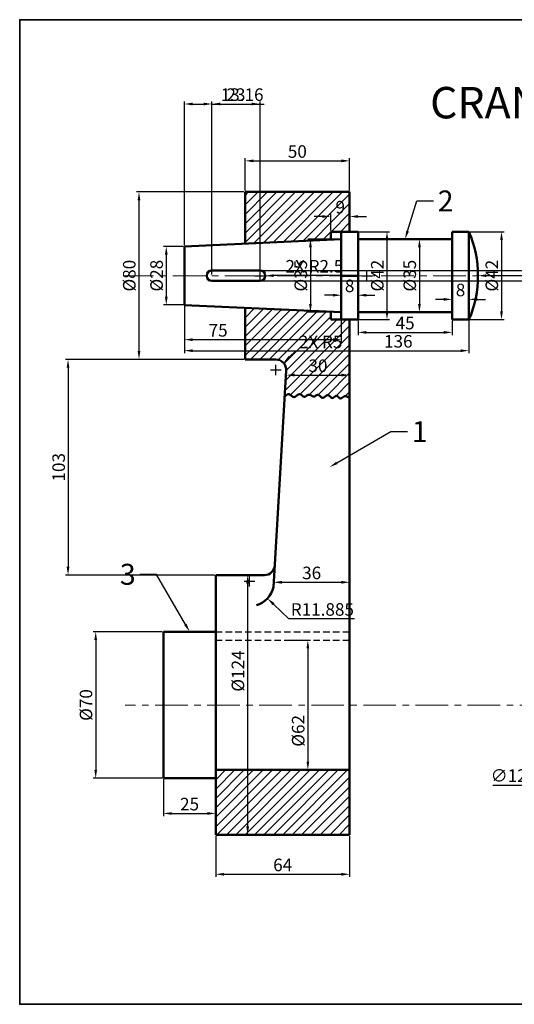
# Model space of a CAD drawing. Units: millimetres. Extents: x -165 to 405, y -25 to 445.
# Tile 1 of 2: x -165 to 72, y -25 to 445. Entities that reach past the tile are written whole.
import ezdxf
from ezdxf import colors
from ezdxf.entities.mleader import LeaderData, LeaderLine
from ezdxf.math import Vec2, Vec3

# ---------------------------------------------------------------- set-up
doc = ezdxf.new("R2010")
doc.units = ezdxf.units.MM
doc.header["$LTSCALE"] = 0.7
doc.linetypes.add('CENTER', pattern=[50.8, 31.75, -6.35, 6.35, -6.35])
doc.linetypes.add('HIDDEN', pattern=[9.525, 6.35, -3.175])
for name, color, linetype, lineweight in [('M-CNTR', 1, 'CENTER', 18), ('M-DIMS', 2, 'Continuous', 25), ('M-HATC', 8, 'Continuous', 18), ('M-HIDN', 6, 'HIDDEN', 25), ('M-OUTL', 7, 'Continuous', 50), ('M-TEXT', 3, 'Continuous', 25), ('M-TTLB', 7, 'Continuous', 35)]:
    doc.layers.add(name, color=color, linetype=linetype, lineweight=lineweight)
doc.styles.get("Standard").update_dxf_attribs({"font": 'arial.ttf'})
doc.dimstyles.new('ISO-25', dxfattribs={"dimtxt": 6, "dimasz": 4, "dimexe": 1.25, "dimexo": 0.625, "dimtad": 1, "dimtoh": 1, "dimdec": 0, "dimtxsty": 'Standard', "dimcen": 2.5, "dimadec": 0, "dimazin": 0, "dimtfac": 1, "dimtdec": 0, "dimtofl": 0, "dimtmove": 0, "dimatfit": 3, "dimfxl": 1, "dimarcsym": 0})

# ---------------------------------------------------------------- blocks, each defined once
blk = doc.blocks.new('*D10')
at = {"layer": 'Defpoints', "color": 0, "ltscale": 0.7, "transparency": 16777216}
for p in [(210.34, 146.19), (100.41, 88.8)]:
    blk.add_point(p, dxfattribs=at)
at = {"layer": 'M-DIMS', "color": 0, "lineweight": -2, "ltscale": 0.7, "transparency": 16777216}
for p, q in [((155.38, 115), (155.38, 120)), ((152.88, 117.5), (157.88, 117.5)), ((81.97, 79.17), (96.87, 86.95)), ((61.58, 79.17), (81.97, 79.17))]:
    blk.add_line(p, q, dxfattribs=at)
at = {"layer": 'M-DIMS', "color": 0, "ltscale": 0.7, "transparency": 16777216}
blk.add_solid([(96.56, 87.54), (97.18, 86.36), (100.41, 88.8)], dxfattribs=at)
at = {"layer": 'M-DIMS', "color": 0, "ltscale": 0.7, "transparency": 16777216, "insert": (71.46, 83.03), "char_height": 6, "attachment_point": 5}
blk.add_mtext('∅124', dxfattribs=at)
blk = doc.blocks.new('*D14')
at = {"layer": 'Defpoints', "color": 0, "ltscale": 0.7, "transparency": 16777216}
for p in [(-95.82, 152.5), (-128.19, 82.5), (-95.82, 82.5)]:
    blk.add_point(p, dxfattribs=at)
at = {"layer": 'M-DIMS', "color": 0, "lineweight": -2, "ltscale": 0.7, "transparency": 16777216}
for p, q in [((-96.44, 152.5), (-129.44, 152.5)), ((-128.19, 148.5), (-128.19, 86.5)), ((-96.44, 82.5), (-129.44, 82.5))]:
    blk.add_line(p, q, dxfattribs=at)
at = {"layer": 'M-DIMS', "color": 0, "ltscale": 0.7, "transparency": 16777216}
for points in [[(-128.86, 148.5), (-127.53, 148.5), (-128.19, 152.5)], [(-128.86, 86.5), (-127.53, 86.5), (-128.19, 82.5)]]:
    blk.add_solid(points, dxfattribs=at)
at = {"layer": 'M-DIMS', "color": 0, "ltscale": 0.7, "transparency": 16777216, "insert": (-132.05, 117.5), "char_height": 6, "attachment_point": 5, "rotation": 90}
blk.add_mtext('%%C70', dxfattribs=at)
blk = doc.blocks.new('*D15')
at = {"layer": 'Defpoints', "color": 0, "ltscale": 0.7, "transparency": 16777216}
for p in [(-95.82, 82.5), (-70.82, 82.5), (-70.82, 65.72)]:
    blk.add_point(p, dxfattribs=at)
at = {"layer": 'M-DIMS', "color": 0, "lineweight": -2, "ltscale": 0.7, "transparency": 16777216}
for p, q in [((-95.82, 81.87), (-95.82, 64.47)), ((-70.82, 81.87), (-70.82, 64.47)), ((-91.82, 65.72), (-74.82, 65.72))]:
    blk.add_line(p, q, dxfattribs=at)
at = {"layer": 'M-DIMS', "color": 0, "ltscale": 0.7, "transparency": 16777216}
for points in [[(-91.82, 66.38), (-91.82, 65.05), (-95.82, 65.72)], [(-74.82, 66.38), (-74.82, 65.05), (-70.82, 65.72)]]:
    blk.add_solid(points, dxfattribs=at)
at = {"layer": 'M-DIMS', "color": 0, "ltscale": 0.7, "transparency": 16777216, "insert": (-83.32, 69.4), "char_height": 6, "attachment_point": 5}
blk.add_mtext('25', dxfattribs=at)
blk = doc.blocks.new('*D16')
at = {"layer": 'Defpoints', "color": 0, "ltscale": 0.7, "transparency": 16777216}
for p in [(-70.82, 55.5), (-6.82, 55.5), (-6.82, 36.67)]:
    blk.add_point(p, dxfattribs=at)
at = {"layer": 'M-DIMS', "color": 0, "lineweight": -2, "ltscale": 0.7, "transparency": 16777216}
for p, q in [((-70.82, 54.87), (-70.82, 35.42)), ((-6.82, 54.87), (-6.82, 35.42)), ((-66.82, 36.67), (-10.82, 36.67))]:
    blk.add_line(p, q, dxfattribs=at)
at = {"layer": 'M-DIMS', "color": 0, "ltscale": 0.7, "transparency": 16777216}
for points in [[(-66.82, 37.34), (-66.82, 36.01), (-70.82, 36.67)], [(-10.82, 37.34), (-10.82, 36.01), (-6.82, 36.67)]]:
    blk.add_solid(points, dxfattribs=at)
at = {"layer": 'M-DIMS', "color": 0, "ltscale": 0.7, "transparency": 16777216, "insert": (-38.82, 40.36), "char_height": 6, "attachment_point": 5}
blk.add_mtext('64', dxfattribs=at)
blk = doc.blocks.new('*D17')
at = {"layer": 'Defpoints', "color": 0, "ltscale": 0.7, "transparency": 16777216}
for p in [(-59.17, 179.5), (-59.17, 55.5), (-55.59, 55.5)]:
    blk.add_point(p, dxfattribs=at)
at = {"layer": 'M-DIMS', "color": 0, "lineweight": -2, "ltscale": 0.7, "transparency": 16777216}
for p, q in [((-58.55, 179.5), (-54.34, 179.5)), ((-55.59, 175.5), (-55.59, 59.5)), ((-58.55, 55.5), (-54.34, 55.5))]:
    blk.add_line(p, q, dxfattribs=at)
at = {"layer": 'M-DIMS', "color": 0, "ltscale": 0.7, "transparency": 16777216}
for points in [[(-56.25, 175.5), (-54.92, 175.5), (-55.59, 179.5)], [(-56.25, 59.5), (-54.92, 59.5), (-55.59, 55.5)]]:
    blk.add_solid(points, dxfattribs=at)
at = {"layer": 'M-DIMS', "color": 0, "ltscale": 0.7, "transparency": 16777216, "insert": (-59.44, 133.73), "char_height": 6, "attachment_point": 5, "rotation": 90}
blk.add_mtext('%%C124', dxfattribs=at)
blk = doc.blocks.new('*D18')
at = {"layer": 'Defpoints', "color": 0, "ltscale": 0.7, "transparency": 16777216}
for p in [(-38.82, 148.5), (-38.82, 86.5), (-26.79, 86.5)]:
    blk.add_point(p, dxfattribs=at)
at = {"layer": 'M-DIMS', "color": 0, "lineweight": -2, "ltscale": 0.7, "transparency": 16777216}
for p, q in [((-38.19, 148.5), (-25.54, 148.5)), ((-26.79, 144.5), (-26.79, 90.5)), ((-38.19, 86.5), (-25.54, 86.5))]:
    blk.add_line(p, q, dxfattribs=at)
at = {"layer": 'M-DIMS', "color": 0, "ltscale": 0.7, "transparency": 16777216}
for points in [[(-27.45, 144.5), (-26.12, 144.5), (-26.79, 148.5)], [(-27.45, 90.5), (-26.12, 90.5), (-26.79, 86.5)]]:
    blk.add_solid(points, dxfattribs=at)
at = {"layer": 'M-DIMS', "color": 0, "ltscale": 0.7, "transparency": 16777216, "insert": (-30.64, 105.17), "char_height": 6, "attachment_point": 5, "rotation": 90}
blk.add_mtext('%%C62', dxfattribs=at)
blk = doc.blocks.new('*D19')
at = {"layer": 'Defpoints', "color": 0, "ltscale": 0.7, "transparency": 16777216}
for p in [(-6.82, 176.09), (-43.15, 173.79), (-6.82, 173.79)]:
    blk.add_point(p, dxfattribs=at)
at = {"layer": 'M-DIMS', "color": 0, "lineweight": -2, "ltscale": 0.7, "transparency": 16777216}
for p, q in [((-43.15, 174.41), (-43.15, 177.34)), ((-39.15, 176.09), (-10.82, 176.09)), ((-6.82, 174.41), (-6.82, 177.34))]:
    blk.add_line(p, q, dxfattribs=at)
at = {"layer": 'M-DIMS', "color": 0, "ltscale": 0.7, "transparency": 16777216}
for points in [[(-39.15, 176.76), (-39.15, 175.42), (-43.15, 176.09)], [(-10.82, 176.76), (-10.82, 175.42), (-6.82, 176.09)]]:
    blk.add_solid(points, dxfattribs=at)
at = {"layer": 'M-DIMS', "color": 0, "ltscale": 0.7, "transparency": 16777216, "insert": (-24.98, 179.78), "char_height": 6, "attachment_point": 5}
blk.add_mtext('36', dxfattribs=at)
blk = doc.blocks.new('*D20')
at = {"layer": 'Defpoints', "color": 0, "ltscale": 0.7, "transparency": 16777216}
for p in [(-37.12, 277.21), (-6.82, 277.21), (-6.82, 275.03)]:
    blk.add_point(p, dxfattribs=at)
at = {"layer": 'M-DIMS', "color": 0, "lineweight": -2, "ltscale": 0.7, "transparency": 16777216}
for p, q in [((-37.12, 276.58), (-37.12, 273.78)), ((-33.12, 275.03), (-10.82, 275.03)), ((-6.82, 276.58), (-6.82, 273.78))]:
    blk.add_line(p, q, dxfattribs=at)
at = {"layer": 'M-DIMS', "color": 0, "ltscale": 0.7, "transparency": 16777216}
for points in [[(-33.12, 275.7), (-33.12, 274.36), (-37.12, 275.03)], [(-10.82, 275.7), (-10.82, 274.36), (-6.82, 275.03)]]:
    blk.add_solid(points, dxfattribs=at)
at = {"layer": 'M-DIMS', "color": 0, "ltscale": 0.7, "transparency": 16777216, "insert": (-21.97, 278.72), "char_height": 6, "attachment_point": 5}
blk.add_mtext('30', dxfattribs=at)
blk = doc.blocks.new('*D21')
at = {"layer": 'Defpoints', "color": 0, "ltscale": 0.7, "transparency": 16777216}
for p in [(-85.82, 336.5), (-94.46, 308.5), (-85.82, 308.5)]:
    blk.add_point(p, dxfattribs=at)
at = {"layer": 'M-DIMS', "color": 0, "lineweight": -2, "ltscale": 0.7, "transparency": 16777216}
for p, q in [((-86.44, 336.5), (-95.71, 336.5)), ((-94.46, 332.5), (-94.46, 312.5)), ((-86.44, 308.5), (-95.71, 308.5))]:
    blk.add_line(p, q, dxfattribs=at)
at = {"layer": 'M-DIMS', "color": 0, "ltscale": 0.7, "transparency": 16777216}
for points in [[(-95.13, 332.5), (-93.79, 332.5), (-94.46, 336.5)], [(-95.13, 312.5), (-93.79, 312.5), (-94.46, 308.5)]]:
    blk.add_solid(points, dxfattribs=at)
at = {"layer": 'M-DIMS', "color": 0, "ltscale": 0.7, "transparency": 16777216, "insert": (-98.32, 322.5), "char_height": 6, "attachment_point": 5, "rotation": 90}
blk.add_mtext('%%C28', dxfattribs=at)
blk = doc.blocks.new('*D22')
at = {"layer": 'Defpoints', "color": 0, "ltscale": 0.7, "transparency": 16777216}
for p in [(-56.82, 362.5), (-107.5, 282.5), (-56.82, 282.5)]:
    blk.add_point(p, dxfattribs=at)
at = {"layer": 'M-DIMS', "color": 0, "lineweight": -2, "ltscale": 0.7, "transparency": 16777216}
for p, q in [((-57.44, 362.5), (-108.75, 362.5)), ((-107.5, 358.5), (-107.5, 286.5)), ((-57.44, 282.5), (-108.75, 282.5))]:
    blk.add_line(p, q, dxfattribs=at)
at = {"layer": 'M-DIMS', "color": 0, "ltscale": 0.7, "transparency": 16777216}
for points in [[(-108.17, 358.5), (-106.83, 358.5), (-107.5, 362.5)], [(-108.17, 286.5), (-106.83, 286.5), (-107.5, 282.5)]]:
    blk.add_solid(points, dxfattribs=at)
at = {"layer": 'M-DIMS', "color": 0, "ltscale": 0.7, "transparency": 16777216, "insert": (-111.36, 322.5), "char_height": 6, "attachment_point": 5, "rotation": 90}
blk.add_mtext('%%C80', dxfattribs=at)
blk = doc.blocks.new('*D23')
at = {"layer": 'Defpoints', "color": 0, "ltscale": 0.7, "transparency": 16777216}
for p in [(-6.82, 377.32), (-56.82, 362.5), (-6.82, 362.5)]:
    blk.add_point(p, dxfattribs=at)
at = {"layer": 'M-DIMS', "color": 0, "lineweight": -2, "ltscale": 0.7, "transparency": 16777216}
for p, q in [((-56.82, 363.12), (-56.82, 378.57)), ((-52.82, 377.32), (-10.82, 377.32)), ((-6.82, 363.12), (-6.82, 378.57))]:
    blk.add_line(p, q, dxfattribs=at)
at = {"layer": 'M-DIMS', "color": 0, "ltscale": 0.7, "transparency": 16777216}
for points in [[(-52.82, 377.99), (-52.82, 376.65), (-56.82, 377.32)], [(-10.82, 377.99), (-10.82, 376.65), (-6.82, 377.32)]]:
    blk.add_solid(points, dxfattribs=at)
at = {"layer": 'M-DIMS', "color": 0, "ltscale": 0.7, "transparency": 16777216, "insert": (-31.82, 381.01), "char_height": 6, "attachment_point": 5}
blk.add_mtext('50', dxfattribs=at)
blk = doc.blocks.new('*D24')
at = {"layer": 'Defpoints', "color": 0, "ltscale": 0.7, "transparency": 16777216}
for p in [(-6.82, 350.75), (-15.82, 343.5), (-6.82, 343.5)]:
    blk.add_point(p, dxfattribs=at)
at = {"layer": 'M-DIMS', "color": 0, "lineweight": -2, "ltscale": 0.7, "transparency": 16777216}
for p, q in [((-19.82, 350.75), (-23.82, 350.75)), ((-15.82, 344.12), (-15.82, 352)), ((-6.82, 344.12), (-6.82, 352)), ((-2.82, 350.75), (1.18, 350.75))]:
    blk.add_line(p, q, dxfattribs=at)
at = {"layer": 'M-DIMS', "color": 0, "ltscale": 0.7, "transparency": 16777216}
for points in [[(-19.82, 351.42), (-19.82, 350.09), (-15.82, 350.75)], [(-2.82, 351.42), (-2.82, 350.09), (-6.82, 350.75)]]:
    blk.add_solid(points, dxfattribs=at)
at = {"layer": 'M-DIMS', "color": 0, "ltscale": 0.7, "transparency": 16777216, "insert": (-11.32, 354.44), "char_height": 6, "attachment_point": 5}
blk.add_mtext('9', dxfattribs=at)
blk = doc.blocks.new('*D25')
at = {"layer": 'Defpoints', "color": 0, "ltscale": 0.7, "transparency": 16777216}
for p in [(-85.82, 308.5), (-10.82, 301.5), (-10.82, 291.95)]:
    blk.add_point(p, dxfattribs=at)
at = {"layer": 'M-DIMS', "color": 0, "lineweight": -2, "ltscale": 0.7, "transparency": 16777216}
for p, q in [((-85.82, 307.87), (-85.82, 290.7)), ((-10.82, 300.87), (-10.82, 290.7)), ((-81.82, 291.95), (-14.82, 291.95))]:
    blk.add_line(p, q, dxfattribs=at)
at = {"layer": 'M-DIMS', "color": 0, "ltscale": 0.7, "transparency": 16777216}
for points in [[(-81.82, 292.61), (-81.82, 291.28), (-85.82, 291.95)], [(-14.82, 292.61), (-14.82, 291.28), (-10.82, 291.95)]]:
    blk.add_solid(points, dxfattribs=at)
at = {"layer": 'M-DIMS', "color": 0, "ltscale": 0.7, "transparency": 16777216, "insert": (-69.68, 295.62), "char_height": 6, "attachment_point": 5}
blk.add_mtext('75', dxfattribs=at)
blk = doc.blocks.new('*D26')
at = {"layer": 'Defpoints', "color": 0, "ltscale": 0.7, "transparency": 16777216}
for p in [(-85.82, 322.5), (50.18, 322.5), (50.18, 286.68)]:
    blk.add_point(p, dxfattribs=at)
at = {"layer": 'M-DIMS', "color": 0, "lineweight": -2, "ltscale": 0.7, "transparency": 16777216}
for p, q in [((-85.82, 321.87), (-85.82, 285.43)), ((50.18, 321.87), (50.18, 285.43)), ((-81.82, 286.68), (46.18, 286.68))]:
    blk.add_line(p, q, dxfattribs=at)
at = {"layer": 'M-DIMS', "color": 0, "ltscale": 0.7, "transparency": 16777216}
for points in [[(-81.82, 287.35), (-81.82, 286.01), (-85.82, 286.68)], [(46.18, 287.35), (46.18, 286.01), (50.18, 286.68)]]:
    blk.add_solid(points, dxfattribs=at)
at = {"layer": 'M-DIMS', "color": 0, "ltscale": 0.7, "transparency": 16777216, "insert": (16.44, 290.37), "char_height": 6, "attachment_point": 5}
blk.add_mtext('136', dxfattribs=at)
blk = doc.blocks.new('*D27')
at = {"layer": 'Defpoints', "color": 0, "ltscale": 0.7, "transparency": 16777216}
for p in [(-10.82, 343.5), (-6.82, 301.5), (11.03, 301.5)]:
    blk.add_point(p, dxfattribs=at)
at = {"layer": 'M-DIMS', "color": 0, "lineweight": -2, "ltscale": 0.7, "transparency": 16777216}
for p, q in [((-10.19, 343.5), (12.28, 343.5)), ((11.03, 339.5), (11.03, 305.5)), ((-6.19, 301.5), (12.28, 301.5))]:
    blk.add_line(p, q, dxfattribs=at)
at = {"layer": 'M-DIMS', "color": 0, "ltscale": 0.7, "transparency": 16777216}
for points in [[(10.36, 339.5), (11.69, 339.5), (11.03, 343.5)], [(10.36, 305.5), (11.69, 305.5), (11.03, 301.5)]]:
    blk.add_solid(points, dxfattribs=at)
at = {"layer": 'M-DIMS', "color": 0, "ltscale": 0.7, "transparency": 16777216, "insert": (7.17, 322.5), "char_height": 6, "attachment_point": 5, "rotation": 90}
blk.add_mtext('%%C42', dxfattribs=at)
blk = doc.blocks.new('*D28')
at = {"layer": 'Defpoints', "color": 0, "ltscale": 0.7, "transparency": 16777216}
for p in [(-10.82, 313.17), (-2.82, 313.17), (-2.82, 313.17)]:
    blk.add_point(p, dxfattribs=at)
at = {"layer": 'M-DIMS', "color": 0, "lineweight": -2, "ltscale": 0.7, "transparency": 16777216}
for p, q in [((-14.82, 313.17), (-18.82, 313.17)), ((-10.82, 313.8), (-10.82, 314.42)), ((-2.82, 313.8), (-2.82, 314.42)), ((1.18, 313.17), (5.18, 313.17))]:
    blk.add_line(p, q, dxfattribs=at)
at = {"layer": 'M-DIMS', "color": 0, "ltscale": 0.7, "transparency": 16777216}
for points in [[(-14.82, 313.84), (-14.82, 312.51), (-10.82, 313.17)], [(1.18, 313.84), (1.18, 312.51), (-2.82, 313.17)]]:
    blk.add_solid(points, dxfattribs=at)
at = {"layer": 'M-DIMS', "color": 0, "ltscale": 0.7, "transparency": 16777216, "insert": (-6.82, 316.86), "char_height": 6, "attachment_point": 5}
blk.add_mtext('8', dxfattribs=at)
blk = doc.blocks.new('*D29')
at = {"layer": 'Defpoints', "color": 0, "ltscale": 0.7, "transparency": 16777216}
for p in [(-10.82, 340), (-25.55, 305), (-10.82, 305)]:
    blk.add_point(p, dxfattribs=at)
at = {"layer": 'M-DIMS', "color": 0, "lineweight": -2, "ltscale": 0.7, "transparency": 16777216}
for p, q in [((-11.44, 340), (-26.8, 340)), ((-25.55, 336), (-25.55, 309)), ((-11.44, 305), (-26.8, 305))]:
    blk.add_line(p, q, dxfattribs=at)
at = {"layer": 'M-DIMS', "color": 0, "ltscale": 0.7, "transparency": 16777216}
for points in [[(-26.22, 336), (-24.89, 336), (-25.55, 340)], [(-26.22, 309), (-24.89, 309), (-25.55, 305)]]:
    blk.add_solid(points, dxfattribs=at)
at = {"layer": 'M-DIMS', "color": 0, "ltscale": 0.7, "transparency": 16777216, "insert": (-29.41, 322.5), "char_height": 6, "attachment_point": 5, "rotation": 90}
blk.add_mtext('%%C35', dxfattribs=at)
blk = doc.blocks.new('*D30')
at = {"layer": 'Defpoints', "color": 0, "ltscale": 0.7, "transparency": 16777216}
for p in [(28.45, 340), (26.53, 305), (28.45, 305)]:
    blk.add_point(p, dxfattribs=at)
at = {"layer": 'M-DIMS', "color": 0, "lineweight": -2, "ltscale": 0.7, "transparency": 16777216}
for p, q in [((27.83, 340), (25.28, 340)), ((26.53, 336), (26.53, 309)), ((27.83, 305), (25.28, 305))]:
    blk.add_line(p, q, dxfattribs=at)
at = {"layer": 'M-DIMS', "color": 0, "ltscale": 0.7, "transparency": 16777216}
for points in [[(25.87, 336), (27.2, 336), (26.53, 340)], [(25.87, 309), (27.2, 309), (26.53, 305)]]:
    blk.add_solid(points, dxfattribs=at)
at = {"layer": 'M-DIMS', "color": 0, "ltscale": 0.7, "transparency": 16777216, "insert": (22.68, 322.5), "char_height": 6, "attachment_point": 5, "rotation": 90}
blk.add_mtext('%%C35', dxfattribs=at)
blk = doc.blocks.new('*D31')
at = {"layer": 'Defpoints', "color": 0, "ltscale": 0.7, "transparency": 16777216}
for p in [(46.18, 343.5), (46.18, 301.5), (65.76, 301.5)]:
    blk.add_point(p, dxfattribs=at)
at = {"layer": 'M-DIMS', "color": 0, "lineweight": -2, "ltscale": 0.7, "transparency": 16777216}
for p, q in [((46.81, 343.5), (67.01, 343.5)), ((65.76, 339.5), (65.76, 305.5)), ((46.81, 301.5), (67.01, 301.5))]:
    blk.add_line(p, q, dxfattribs=at)
at = {"layer": 'M-DIMS', "color": 0, "ltscale": 0.7, "transparency": 16777216}
for points in [[(65.1, 339.5), (66.43, 339.5), (65.76, 343.5)], [(65.1, 305.5), (66.43, 305.5), (65.76, 301.5)]]:
    blk.add_solid(points, dxfattribs=at)
at = {"layer": 'M-DIMS', "color": 0, "ltscale": 0.7, "transparency": 16777216, "insert": (61.91, 322.5), "char_height": 6, "attachment_point": 5, "rotation": 90}
blk.add_mtext('%%C42', dxfattribs=at)
blk = doc.blocks.new('*D32')
at = {"layer": 'Defpoints', "color": 0, "ltscale": 0.7, "transparency": 16777216}
for p in [(-2.82, 301.5), (42.18, 301.5), (42.18, 295.42)]:
    blk.add_point(p, dxfattribs=at)
at = {"layer": 'M-DIMS', "color": 0, "lineweight": -2, "ltscale": 0.7, "transparency": 16777216}
for p, q in [((-2.82, 300.87), (-2.82, 294.17)), ((42.18, 300.87), (42.18, 294.17)), ((1.18, 295.42), (38.18, 295.42))]:
    blk.add_line(p, q, dxfattribs=at)
at = {"layer": 'M-DIMS', "color": 0, "ltscale": 0.7, "transparency": 16777216}
for points in [[(1.18, 296.09), (1.18, 294.75), (-2.82, 295.42)], [(38.18, 296.09), (38.18, 294.75), (42.18, 295.42)]]:
    blk.add_solid(points, dxfattribs=at)
at = {"layer": 'M-DIMS', "color": 0, "ltscale": 0.7, "transparency": 16777216, "insert": (19.68, 299.09), "char_height": 6, "attachment_point": 5}
blk.add_mtext('45', dxfattribs=at)
blk = doc.blocks.new('*D33')
at = {"layer": 'Defpoints', "color": 0, "ltscale": 0.7, "transparency": 16777216}
for p in [(50.18, 311.19), (42.18, 301.5), (50.18, 301.5)]:
    blk.add_point(p, dxfattribs=at)
at = {"layer": 'M-DIMS', "color": 0, "lineweight": -2, "ltscale": 0.7, "transparency": 16777216}
for p, q in [((38.18, 311.19), (34.18, 311.19)), ((42.18, 302.12), (42.18, 312.44)), ((50.18, 302.12), (50.18, 312.44)), ((54.18, 311.19), (58.18, 311.19))]:
    blk.add_line(p, q, dxfattribs=at)
at = {"layer": 'M-DIMS', "color": 0, "ltscale": 0.7, "transparency": 16777216}
for points in [[(38.18, 311.86), (38.18, 310.52), (42.18, 311.19)], [(54.18, 311.86), (54.18, 310.52), (50.18, 311.19)]]:
    blk.add_solid(points, dxfattribs=at)
at = {"layer": 'M-DIMS', "color": 0, "ltscale": 0.7, "transparency": 16777216, "insert": (46.18, 314.88), "char_height": 6, "attachment_point": 5}
blk.add_mtext('8', dxfattribs=at)
blk = doc.blocks.new('*D39')
at = {"layer": 'Defpoints', "color": 0, "ltscale": 0.7, "transparency": 16777216}
for p in [(1.44, 322.5), (54.52, 322.5)]:
    blk.add_point(p, dxfattribs=at)
at = {"layer": 'M-DIMS', "color": 0, "lineweight": -2, "ltscale": 0.7, "transparency": 16777216}
for p, q in [((1.44, 320), (1.44, 325)), ((-1.06, 322.5), (3.94, 322.5)), ((86.36, 322.5), (58.52, 322.5)), ((112.99, 322.5), (86.36, 322.5))]:
    blk.add_line(p, q, dxfattribs=at)
at = {"layer": 'M-DIMS', "color": 0, "ltscale": 0.7, "transparency": 16777216}
blk.add_solid([(58.52, 323.16), (58.52, 321.83), (54.52, 322.5)], dxfattribs=at)
at = {"layer": 'M-DIMS', "color": 0, "ltscale": 0.7, "transparency": 16777216, "insert": (99.99, 326.19), "char_height": 6, "attachment_point": 5}
blk.add_mtext('R53.08', dxfattribs=at)
blk = doc.blocks.new('*D40')
at = {"layer": 'Defpoints', "color": 0, "ltscale": 0.7, "transparency": 16777216}
for p in [(-54.7, 176.56), (-46.08, 168.38)]:
    blk.add_point(p, dxfattribs=at)
at = {"layer": 'M-DIMS', "color": 0, "lineweight": -2, "ltscale": 0.7, "transparency": 16777216}
for p, q in [((-54.7, 174.06), (-54.7, 179.06)), ((-57.2, 176.56), (-52.2, 176.56)), ((-35.84, 158.66), (-43.18, 165.63)), ((-4.52, 158.66), (-35.84, 158.66))]:
    blk.add_line(p, q, dxfattribs=at)
at = {"layer": 'M-DIMS', "color": 0, "ltscale": 0.7, "transparency": 16777216}
blk.add_solid([(-42.72, 166.11), (-43.64, 165.14), (-46.08, 168.38)], dxfattribs=at)
at = {"layer": 'M-DIMS', "color": 0, "ltscale": 0.7, "transparency": 16777216, "insert": (-19.86, 162.34), "char_height": 6, "attachment_point": 5}
blk.add_mtext('R11.885', dxfattribs=at)
blk = doc.blocks.new('*D41')
at = {"layer": 'Defpoints', "color": 0, "ltscale": 0.7, "transparency": 16777216}
for p in [(-42.12, 277.5), (-38.48, 280.93)]:
    blk.add_point(p, dxfattribs=at)
at = {"layer": 'M-DIMS', "color": 0, "lineweight": -2, "ltscale": 0.7, "transparency": 16777216}
for p, q in [((-32.66, 286.42), (-35.57, 283.67)), ((-9.32, 286.42), (-32.66, 286.42)), ((-44.62, 277.5), (-39.62, 277.5)), ((-42.12, 275), (-42.12, 280))]:
    blk.add_line(p, q, dxfattribs=at)
at = {"layer": 'M-DIMS', "color": 0, "ltscale": 0.7, "transparency": 16777216}
blk.add_solid([(-36.03, 284.16), (-35.11, 283.19), (-38.48, 280.93)], dxfattribs=at)
at = {"layer": 'M-DIMS', "color": 0, "ltscale": 0.7, "transparency": 16777216, "insert": (-20.68, 290.1), "char_height": 6, "attachment_point": 5}
blk.add_mtext('2X R5', dxfattribs=at)
blk = doc.blocks.new('*D42')
at = {"layer": 'Defpoints', "color": 0, "ltscale": 0.7, "transparency": 16777216}
for p in [(-56.82, 282.5), (-141.41, 179.5), (-70.82, 179.5)]:
    blk.add_point(p, dxfattribs=at)
at = {"layer": 'M-DIMS', "color": 0, "lineweight": -2, "ltscale": 0.7, "transparency": 16777216}
for p, q in [((-57.44, 282.5), (-142.66, 282.5)), ((-141.41, 278.5), (-141.41, 183.5)), ((-71.44, 179.5), (-142.66, 179.5))]:
    blk.add_line(p, q, dxfattribs=at)
at = {"layer": 'M-DIMS', "color": 0, "ltscale": 0.7, "transparency": 16777216}
for points in [[(-142.08, 278.5), (-140.75, 278.5), (-141.41, 282.5)], [(-142.08, 183.5), (-140.75, 183.5), (-141.41, 179.5)]]:
    blk.add_solid(points, dxfattribs=at)
at = {"layer": 'M-DIMS', "color": 0, "ltscale": 0.7, "transparency": 16777216, "insert": (-145.11, 231), "char_height": 6, "attachment_point": 5, "rotation": 90}
blk.add_mtext('103', dxfattribs=at)
blk = doc.blocks.new('*D43')
at = {"layer": 'Defpoints', "color": 0, "ltscale": 0.7, "transparency": 16777216}
for p in [(-49.66, 404.47), (-72.66, 322.5), (-49.66, 322.5)]:
    blk.add_point(p, dxfattribs=at)
at = {"layer": 'M-DIMS', "color": 0, "lineweight": -2, "ltscale": 0.7, "transparency": 16777216}
for p, q in [((-72.66, 323.12), (-72.66, 405.72)), ((-68.66, 404.47), (-53.66, 404.47)), ((-49.66, 323.12), (-49.66, 405.72))]:
    blk.add_line(p, q, dxfattribs=at)
at = {"layer": 'M-DIMS', "color": 0, "ltscale": 0.7, "transparency": 16777216}
for points in [[(-68.66, 405.13), (-68.66, 403.8), (-72.66, 404.47)], [(-53.66, 405.13), (-53.66, 403.8), (-49.66, 404.47)]]:
    blk.add_solid(points, dxfattribs=at)
at = {"layer": 'M-DIMS', "color": 0, "ltscale": 0.7, "transparency": 16777216, "insert": (-61.16, 408.16), "char_height": 6, "attachment_point": 5}
blk.add_mtext('23', dxfattribs=at)
blk = doc.blocks.new('*D44')
at = {"layer": 'Defpoints', "color": 0, "ltscale": 0.7, "transparency": 16777216}
for p in [(-72.66, 404.47), (-85.82, 336.5), (-72.66, 322.5)]:
    blk.add_point(p, dxfattribs=at)
at = {"layer": 'M-DIMS', "color": 0, "lineweight": -2, "ltscale": 0.7, "transparency": 16777216}
for p, q in [((-85.82, 337.12), (-85.82, 405.72)), ((-81.82, 404.47), (-76.66, 404.47)), ((-72.66, 323.12), (-72.66, 405.72)), ((-72.66, 404.47), (-47.73, 404.47))]:
    blk.add_line(p, q, dxfattribs=at)
at = {"layer": 'M-DIMS', "color": 0, "ltscale": 0.7, "transparency": 16777216}
for points in [[(-81.82, 405.13), (-81.82, 403.8), (-85.82, 404.47)], [(-76.66, 405.13), (-76.66, 403.8), (-72.66, 404.47)]]:
    blk.add_solid(points, dxfattribs=at)
at = {"layer": 'M-DIMS', "color": 0, "ltscale": 0.7, "transparency": 16777216, "insert": (-58.19, 408.16), "char_height": 6, "attachment_point": 5}
blk.add_mtext('13.16', dxfattribs=at)
blk = doc.blocks.new('*D45')
at = {"layer": 'Defpoints', "color": 0, "ltscale": 0.7, "transparency": 16777216}
for p in [(-49.66, 325), (-49.66, 320), (403.9, 320)]:
    blk.add_point(p, dxfattribs=at)
at = {"layer": 'M-DIMS', "color": 0, "lineweight": -2, "ltscale": 0.7, "transparency": 16777216}
for p, q in [((403.9, 329), (403.9, 333)), ((-49.03, 325), (405.15, 325)), ((-49.03, 320), (405.15, 320)), ((403.9, 316), (403.9, 312)), ((403.9, 312), (399.29, 312))]:
    blk.add_line(p, q, dxfattribs=at)
at = {"layer": 'M-DIMS', "color": 0, "ltscale": 0.7, "transparency": 16777216}
for points in [[(403.23, 329), (404.56, 329), (403.9, 325)], [(403.23, 316), (404.56, 316), (403.9, 320)]]:
    blk.add_solid(points, dxfattribs=at)
at = {"layer": 'M-DIMS', "color": 0, "ltscale": 0.7, "transparency": 16777216, "insert": (401.28, 315.67), "char_height": 6, "attachment_point": 5}
blk.add_mtext('5', dxfattribs=at)
blk = doc.blocks.new('*D46')
at = {"layer": 'Defpoints', "color": 0, "ltscale": 0.7, "transparency": 16777216}
for p in [(-49.66, 322.5), (-47.16, 322.5)]:
    blk.add_point(p, dxfattribs=at)
at = {"layer": 'M-DIMS', "color": 0, "lineweight": -2, "ltscale": 0.7, "transparency": 16777216}
for p, q in [((-49.66, 320), (-49.66, 325)), ((-52.16, 322.5), (-47.16, 322.5)), ((-39.16, 322.51), (-43.16, 322.51)), ((-8.82, 322.51), (-39.16, 322.51))]:
    blk.add_line(p, q, dxfattribs=at)
at = {"layer": 'M-DIMS', "color": 0, "ltscale": 0.7, "transparency": 16777216}
blk.add_solid([(-43.16, 323.17), (-43.15, 321.84), (-47.16, 322.5)], dxfattribs=at)
at = {"layer": 'M-DIMS', "color": 0, "ltscale": 0.7, "transparency": 16777216, "insert": (-23.68, 326.2), "char_height": 6, "attachment_point": 5}
blk.add_mtext('2X R2.5', dxfattribs=at)

msp = doc.modelspace()

# ---------------------------------------------------------------- hatches: boundary and pattern name
at = {"layer": 'M-HATC', "ltscale": 0.7}
h = msp.add_hatch(dxfattribs=at)
h.set_pattern_fill('ANSI31', color=256)
h.paths.add_polyline_path([(-6.8156, 86.4959), (-70.8156, 86.4959), (-70.8156, 82.4959), (-70.8156, 55.4959), (-6.8156, 55.4959)])
h.paths.add_polyline_path([(-6.8156, 362.4959), (-56.8156, 362.4959), (-56.8156, 337.8492), (-15.8156, 339.7625), (-15.8156, 343.4959), (-10.8156, 343.4959), (-6.8156, 343.4959)])
edge = h.paths.add_edge_path()
edge.add_line((-15.8156, 305.2292), (-56.8156, 307.1425))
edge.add_line((-56.8156, 307.1425), (-56.8156, 282.4959))
edge.add_line((-56.8156, 282.4959), (-42.1153, 282.4959))
edge.add_arc((-42.1153, 277.4959), 5, -3.333851, 90, ccw=False)
edge.add_line((-37.1238, 277.2051), (-37.8464, 264.7996))
edge.add_spline(control_points=[(-37.8464, 264.7996), (-37.167, 265.4518), (-35.6482, 266.9098), (-33.2846, 263.1213), (-30.8198, 267.4001), (-28.5561, 263.5168), (-26.3917, 266.7417), (-24.0231, 263.8639), (-21.8949, 266.6713), (-19.7633, 262.6734), (-17.3242, 266.9021), (-15.1634, 262.8974), (-13.0907, 266.0872), (-11.2117, 262.8862), (-9.2278, 265.6704), (-7.6802, 264.7023), (-6.8156, 264.1614)], knot_values=[0, 0, 0, 0, 2.35416727, 5.26229304, 8.17900958, 10.9256319, 12.99668293, 16.02215644, 17.65243494, 20.64118654, 23.30679757, 26.13184074, 28.11376526, 30.50361657, 32.58014241, 35.20920109, 35.20920109, 35.20920109, 35.20920109], degree=3, periodic=0)
edge.add_line((-6.8156, 264.1614), (-6.8156, 301.4959))
edge.add_line((-6.8156, 301.4959), (-10.8156, 301.4959))
edge.add_line((-10.8156, 301.4959), (-15.8156, 301.4959))
edge.add_line((-15.8156, 301.4959), (-15.8156, 305.2292))

# ---------------------------------------------------------------- linework, layer by layer
at = {"layer": 'M-CNTR', "ltscale": 0.7}
for p, q in [((222.9554, 322.4959), (-115.0149, 322.4959)), ((289.1425, 117.4959), (-114.0701, 117.4959))]:
    msp.add_line(p, q, dxfattribs=at)
at = {"layer": 'M-HIDN', "ltscale": 0.7}
for p, q in [((-70.8156, 152.4959), (-6.8156, 152.4959)), ((-70.8156, 148.4959), (-6.8156, 148.4959))]:
    msp.add_line(p, q, dxfattribs=at)
at = {"layer": 'M-OUTL', "ltscale": 0.7}
for p, q in [((-6.8156, 362.4959), (-56.8156, 362.4959)), ((-56.8156, 362.4959), (-56.8156, 337.8492)), ((-6.8156, 343.4959), (-6.8156, 362.4959)), ((-10.8156, 343.4959), (-15.8156, 343.4959)), ((-15.8156, 343.4959), (-15.8156, 339.7625)), ((-10.8156, 343.4959), (-10.8156, 301.4959)), ((-2.8156, 343.4959), (-10.8156, 343.4959)), ((-2.8156, 301.4959), (-2.8156, 343.4959)), ((42.1844, 343.4959), (42.1844, 301.4959)), ((50.1844, 343.4959), (42.1844, 343.4959)), ((50.1844, 301.4959), (50.1844, 343.4959)), ((-85.8156, 336.4959), (-10.8156, 339.9959)), ((-10.8156, 339.9959), (-10.8156, 304.9959)), ((-2.8156, 339.9959), (-2.8156, 304.9959)), ((42.1844, 339.9959), (-2.8156, 339.9959)), ((42.1844, 304.9959), (42.1844, 339.9959)), ((-85.8156, 308.4959), (-85.8156, 336.4959)), ((-72.6552, 324.9959), (-49.6552, 324.9959)), ((-49.6552, 319.9959), (-72.6552, 319.9959)), ((-10.8156, 322.4959), (-2.8156, 322.4959)), ((-85.8156, 308.4959), (-10.8156, 304.9959)), ((-56.8156, 307.1425), (-56.8156, 282.4959)), ((-15.8156, 301.4959), (-15.8156, 305.2292)), ((-10.8156, 301.4959), (-15.8156, 301.4959)), ((-10.8156, 301.4959), (-2.8156, 301.4959)), ((-6.8156, 301.4959), (-6.8156, 55.4959)), ((-2.8156, 304.9959), (42.1844, 304.9959)), ((42.1844, 301.4959), (50.1844, 301.4959)), ((-56.8156, 282.4959), (-42.1153, 282.4959)), ((-43.1481, 173.7873), (-37.1238, 277.2051)), ((-70.8156, 55.4959), (-70.8156, 179.4959)), ((-70.8156, 179.4959), (-47.5328, 179.4959)), ((-95.8156, 82.4959), (-95.8156, 152.4959)), ((-95.8156, 152.4959), (-70.8156, 152.4959)), ((-70.8156, 152.4959), (-70.8156, 82.4959)), ((-70.8156, 86.4959), (-6.8156, 86.4959)), ((-70.8156, 82.4959), (-95.8156, 82.4959)), ((-6.8156, 55.4959), (-70.8156, 55.4959))]:
    msp.add_line(p, q, dxfattribs=at)
for centre, radius, start, end in [((1.4369, 322.4959), 53.0784, 336.69404, 23.30596), ((-72.6552, 322.4959), 2.5, 90, 270), ((-49.6552, 322.4959), 2.5, 270, 90), ((-42.1153, 277.4959), 5, 356.666149, 90), ((-47.5328, 184.4959), 5, 270, 356.666149), ((-54.7049, 176.5627), 11.8854, 286.496054, 346.496054)]:
    msp.add_arc(centre, radius, start, end, dxfattribs=at)
msp.add_open_spline([(-37.8464, 264.7996), (-37.167, 265.4518), (-35.6482, 266.9098), (-33.2846, 263.1213), (-30.8198, 267.4001), (-28.5561, 263.5168), (-26.3917, 266.7417), (-24.0231, 263.8639), (-21.8949, 266.6713), (-19.7633, 262.6734), (-17.3242, 266.9021), (-15.1634, 262.8974), (-13.0907, 266.0872), (-11.2117, 262.8862), (-9.2278, 265.6704), (-7.6802, 264.7023), (-6.8156, 264.1614)], degree=3, knots=[0, 0, 0, 0, 2.35416727, 5.26229304, 8.17900958, 10.9256319, 12.99668293, 16.02215644, 17.65243494, 20.64118654, 23.30679757, 26.13184074, 28.11376526, 30.50361657, 32.58014241, 35.20920109, 35.20920109, 35.20920109, 35.20920109], dxfattribs=at)
at = {"layer": 'M-TTLB', "ltscale": 0.7}
msp.add_lwpolyline([(377.4977, -25.4135), (-164.5299, -25.4135), (-164.5299, 444.7265), (377.4977, 444.7265)], close=True, dxfattribs=at)

# ---------------------------------------------------------------- texts
at = {"layer": 'M-TEXT', "ltscale": 0.7, "insert": (19.3441, 412.6084), "char_height": 15, "attachment_point": 1}
msp.add_mtext_dynamic_manual_height_columns('\\pxqc;CRANK HANDLE', width=175.058291, gutter_width=12.5, heights=[0], dxfattribs=at)

# ---------------------------------------------------------------- dimensions: what is measured, and where the dimension line sits
at = {"layer": 'M-DIMS', "ltscale": 0.7}
for base, p1, p2, override, picture, middle in [((-72.6552, 404.4666), (-85.8156, 336.4959), (-72.6552, 322.4959), {"dimdec": 2, "dimlfac": 1, "dimrnd": 0, "dimzin": 0, "dimdsep": 46, "dimlunit": 2}, '*D44', (-58.1912, 408.157)), ((-49.6552, 404.4666), (-72.6552, 322.4959), (-49.6552, 322.4959), {"dimdec": 0, "dimlfac": 1, "dimrnd": 0, "dimzin": 0, "dimdsep": 46, "dimlunit": 2}, '*D43', (-61.1552, 408.157)), ((-6.8156, 377.3198), (-56.8156, 362.4959), (-6.8156, 362.4959), {"dimclrd": 0, "dimclre": 0, "dimclrt": 0}, '*D23', (-31.8156, 381.0082)), ((-6.8156, 350.7518), (-15.8156, 343.4959), (-6.8156, 343.4959), {"dimclrd": 0, "dimclre": 0, "dimclrt": 0}, '*D24', (-11.3156, 354.4402)), ((-2.8156, 313.1737), (-10.8156, 313.1737), (-2.8156, 313.1737), {"dimclrd": 0, "dimclre": 0, "dimclrt": 0}, '*D28', (-6.8156, 316.8621)), ((50.1844, 311.1891), (42.1844, 301.4959), (50.1844, 301.4959), {"dimclrd": 0, "dimclre": 0, "dimclrt": 0}, '*D33', (46.1844, 314.8776)), ((42.1844, 295.4184), (-2.8156, 301.4959), (42.1844, 301.4959), {"dimclrd": 0, "dimclre": 0, "dimclrt": 0}, '*D32', (19.6844, 299.0946)), ((-6.8156, 275.0294), (-37.1238, 277.2051), (-6.8156, 277.2051), {"dimclrd": 0, "dimclre": 0, "dimclrt": 0}, '*D20', (-21.9697, 278.7199)), ((-6.8156, 176.0885), (-43.1481, 173.7873), (-6.8156, 173.7873), {"dimclrd": 0, "dimclre": 0, "dimclrt": 0}, '*D19', (-24.9819, 179.779)), ((-70.8156, 65.716), (-95.8156, 82.4959), (-70.8156, 82.4959), {"dimclrd": 0, "dimclre": 0, "dimclrt": 0}, '*D15', (-83.3156, 69.4045)), ((-6.8156, 36.6735), (-70.8156, 55.4959), (-6.8156, 55.4959), {"dimclrd": 0, "dimclre": 0, "dimclrt": 0}, '*D16', (-38.8156, 40.3619))]:
    dim = msp.add_linear_dim(base=base, p1=p1, p2=p2, dimstyle='ISO-25', override=override, dxfattribs=at)
    dim.commit()
    dim.dimension.update_dxf_attribs({"geometry": picture, "text_midpoint": middle})
for base, p1, p2, picture, middle in [((-107.4989, 282.4959), (-56.8156, 362.4959), (-56.8156, 282.4959), '*D22', (-111.3551, 322.4959)), ((65.7637, 301.4959), (46.1844, 343.4959), (46.1844, 301.4959), '*D31', (61.9075, 322.4959)), ((-25.5549, 304.9959), (-10.8156, 339.9959), (-10.8156, 304.9959), '*D29', (-29.4111, 322.4959)), ((26.535, 304.9959), (28.4549, 339.9959), (28.4549, 304.9959), '*D30', (22.6787, 322.4959)), ((-94.4591, 308.4959), (-85.8156, 336.4959), (-85.8156, 308.4959), '*D21', (-98.3153, 322.4959)), ((-128.1935, 82.4959), (-95.8156, 152.4959), (-95.8156, 82.4959), '*D14', (-132.0498, 117.4959))]:
    dim = msp.add_linear_dim(base=base, p1=p1, p2=p2, angle=90, text='%%C<>', dimstyle='ISO-25', override={"dimclrd": 0, "dimclre": 0, "dimclrt": 0}, dxfattribs=at)
    dim.commit()
    dim.dimension.update_dxf_attribs({"geometry": picture, "text_midpoint": middle})
for base, p1, p2, picture, middle in [((11.0259, 301.4959), (-10.8156, 343.4959), (-6.8156, 301.4959), '*D27', (7.1697, 322.4959)), ((-55.5883, 55.4959), (-59.1742, 179.4959), (-59.1742, 55.4959), '*D17', (-59.4445, 133.7256)), ((-26.7855, 86.4959), (-38.8156, 148.4959), (-38.8156, 86.4959), '*D18', (-30.6417, 105.1725))]:
    dim = msp.add_linear_dim(base=base, p1=p1, p2=p2, angle=90, text='%%C<>', dimstyle='ISO-25', override={"dimclrd": 0, "dimclre": 0, "dimclrt": 0, "dimtmove": 2}, dxfattribs=at)
    dim.commit()
    dim.dimension.update_dxf_attribs({"geometry": picture, "text_midpoint": middle, "dimtype": 160})
for center, mpoint, override, picture, middle in [((-49.6552, 322.4959), (-47.1552, 322.4999), {"dimdec": 1, "dimlfac": 1, "dimrnd": 0, "dimzin": 0, "dimdsep": 46, "dimlunit": 2}, '*D46', (-23.6775, 326.2013)), ((-42.1153, 277.4959), (-38.4782, 280.9268), {"dimdec": 0, "dimlfac": 1, "dimrnd": 0, "dimzin": 0, "dimdsep": 46, "dimlunit": 2}, '*D41', (-20.6764, 290.1048))]:
    dim = msp.add_radius_dim(center=center, mpoint=mpoint, text='2X <>', dimstyle='ISO-25', override=override, dxfattribs=at)
    dim.commit()
    dim.dimension.update_dxf_attribs({"geometry": picture, "text_midpoint": middle})
for base, p1, p2, picture, middle in [((403.8977, 319.9959), (-49.6552, 324.9959), (-49.6552, 319.9959), '*D45', (401.2836, 315.672)), ((-141.4149, 179.4959), (-56.8156, 282.4959), (-70.8156, 179.4959), '*D42', (-145.1054, 230.9959))]:
    dim = msp.add_linear_dim(base=base, p1=p1, p2=p2, angle=90, dimstyle='ISO-25', override={"dimdec": 0, "dimlfac": 1, "dimrnd": 0, "dimzin": 0, "dimdsep": 46, "dimlunit": 2}, dxfattribs=at)
    dim.commit()
    dim.dimension.update_dxf_attribs({"geometry": picture, "text_midpoint": middle})
dim = msp.add_radius_dim(center=(1.4369, 322.4959), mpoint=(54.5153, 322.496), dimstyle='ISO-25', override={"dimdec": 2, "dimlfac": 1, "dimrnd": 0, "dimzin": 0, "dimdsep": 46, "dimlunit": 2}, dxfattribs=at)
dim.commit()
dim.dimension.update_dxf_attribs({"geometry": '*D39', "text_midpoint": (86.3624, 322.4961), "dimtype": 164})
for base, p1, p2, picture, middle in [((50.1844, 286.6792), (-85.8156, 322.4959), (50.1844, 322.4959), '*D26', (16.4391, 290.3697)), ((-10.8156, 291.9465), (-85.8156, 308.4959), (-10.8156, 301.4959), '*D25', (-69.6845, 295.6227))]:
    dim = msp.add_linear_dim(base=base, p1=p1, p2=p2, dimstyle='ISO-25', override={"dimclrd": 0, "dimclre": 0, "dimclrt": 0, "dimtmove": 2}, dxfattribs=at)
    dim.commit()
    dim.dimension.update_dxf_attribs({"geometry": picture, "text_midpoint": middle, "dimtype": 160})
dim = msp.add_radius_dim(center=(-54.7049, 176.5627), mpoint=(-46.084, 168.381), dimstyle='ISO-25', override={"dimdec": 3, "dimlfac": 1, "dimrnd": 0, "dimzin": 0, "dimdsep": 46, "dimlunit": 2}, dxfattribs=at)
dim.commit()
dim.dimension.update_dxf_attribs({"geometry": '*D40', "text_midpoint": (-19.8643, 162.3446)})
dim = msp.add_diameter_dim_2p(p1=(210.3382, 146.1873), p2=(100.4146, 88.8045), dimstyle='ISO-25', override={"dimclrd": 0, "dimclre": 0, "dimclrt": 0}, dxfattribs=at)
dim.commit()
dim.dimension.update_dxf_attribs({"geometry": '*D10', "text_midpoint": (71.4608, 79.1737), "dimtype": 163})

# ---------------------------------------------------------------- leaders
ml = msp.add_multileader_mtext('Standard', dxfattribs=at)
ml.set_content('2', color=256)
ml.set_leader_properties()
ml.build(insert=Vec2(0, 0))
ctx = ml.context
ctx.base_point, ctx.char_height, ctx.plane_origin = Vec3(33.2705, 358.1686), 10, Vec3(19.6844, 339.9959)
notes = []
notes.append((ctx, [(0, (1, 1, 0), (25.2705, 358.1686), (1, 0), 8, [(0, [(19.6844, 339.9959)], 0, [])])]))
ctx.mtext.insert, ctx.mtext.flow_direction = Vec3(35.2705, 363.1686), 5
ml = msp.add_multileader_mtext('Standard', dxfattribs=at)
ml.set_content('1', color=256)
ml.set_leader_properties()
ml.build(insert=Vec2(0, 0))
ctx = ml.context
ctx.base_point, ctx.char_height, ctx.plane_origin = Vec3(20.8785, 248.0163), 10, Vec3(-16.4011, 231.1117)
notes.append((ctx, [(0, (1, 1, 0), (12.8785, 248.0163), (1, 0), 8, [(0, [(-16.4011, 231.1117)], 0, [])])]))
ctx.mtext.insert, ctx.mtext.flow_direction = Vec3(22.8785, 253.0163), 5
ml = msp.add_multileader_mtext('Standard', dxfattribs=at)
ml.set_content('3', color=256)
ml.set_leader_properties()
ml.build(insert=Vec2(0, 0))
ctx = ml.context
ctx.base_point, ctx.char_height, ctx.plane_origin = Vec3(-117.6396, 179.8199), 10, Vec3(-83.3156, 152.4959)
ctx.text_align_type = 2
notes.append((ctx, [(0, (1, 1, 0), (-99.0911, 179.8199), (-1, 0), 8, [(0, [(-83.3156, 152.4959)], 0, [])])]))
ctx.mtext.insert, ctx.mtext.alignment, ctx.mtext.flow_direction = Vec3(-109.0911, 184.9086), 3, 5
for ctx, leaders in notes:
    for number, flags, end, landing, length, lines in leaders:
        leader = LeaderData()
        leader.index, (leader.has_last_leader_line, leader.has_dogleg_vector, leader.attachment_direction) = number, flags
        leader.last_leader_point, leader.dogleg_vector, leader.dogleg_length = Vec3(end), Vec3(landing), length
        for number, points, colour, breaks in lines:
            line = LeaderLine()
            line.index, line.vertices, line.color, line.breaks = number, Vec3.list(points), colors.encode_raw_color(colour), breaks
            leader.lines.append(line)
        ctx.leaders.append(leader)

doc.saveas('drawing.dxf')
